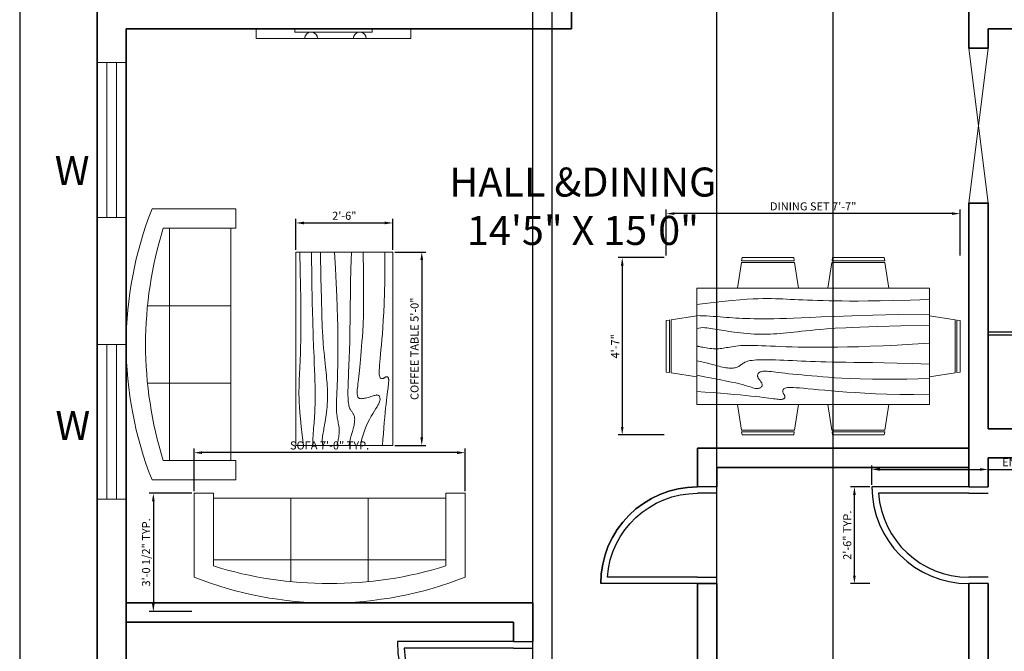
# Model space of a CAD drawing. Units: inches. Extents: x 1868 to 2413, y 1522 to 2138.
# Tile 2 of 4: x 1902 to 2207, y 1727 to 1923. Entities that reach past the tile are written whole.
import ezdxf

# ---------------------------------------------------------------- set-up
doc = ezdxf.new("R2010")
doc.units = ezdxf.units.IN
for name, color, linetype, lineweight in [('A-ANNO-DIMS', 2, 'Continuous', 18), ('A-ANNO-TEXT', 7, 'Continuous', 18), ('A-AREA-IDEN', 7, 'Continuous', 25), ('A-DOOR', 3, 'Continuous', 25), ('A-EQPM', 8, 'Continuous', 18), ('A-FLOR-CASE', 8, 'Continuous', 25), ('A-FLOR-OPEN', 4, 'Continuous', 18), ('A-FURN', 8, 'Continuous', 18), ('A-GLAZ', 4, 'Continuous', 18), ('A-WALL', 7, 'Continuous', 35), ('C-PROP', 7, 'Continuous', 25)]:
    doc.layers.add(name, color=color, linetype=linetype, lineweight=lineweight)
doc.styles.get("Standard").update_dxf_attribs({"font": 'arial.ttf'})
doc.dimstyles.new('ISO-25', dxfattribs={"dimtxt": 2.5, "dimasz": 2.5, "dimexe": 1.25, "dimexo": 0.625, "dimtad": 1, "dimdec": 0, "dimlunit": 3, "dimtxsty": 'Standard', "dimcen": 2.5, "dimadec": 0, "dimazin": 0, "dimtfac": 1, "dimtdec": 0, "dimtmove": 0, "dimatfit": 3, "dimfxl": 1, "dimarcsym": 0})

# ---------------------------------------------------------------- blocks, each defined once
blk = doc.blocks.new('Sofa - Roundback 7 ft.')
for p, q in [((-12.00002, -32.4421), (-12.00003, -6.5971)), ((11.99997, -32.4421), (11.99998, -6.5971)), ((-36.000027, -34), (-36.000027, -11.4696)), ((35.99998, -34), (35.99998, -11.4696)), ((-35.999844, -13.3819), (35.9998, -13.3819)), ((-36.000027, -32.4421), (35.99998, -32.4421))]:
    blk.add_line(p, q)
for points in [[(-36.000027, -34), (-42.000027, -34), (-42.000027, -8)], [(41.99998, -8), (41.99998, -34), (35.99998, -34)]]:
    blk.add_lwpolyline(points)
for centre, radius, start, end in [((0, -114.25), 114.25, 68.43141, 111.5686), ((-0.00001, -127.1968), 121.1968, 72.72033, 107.2797)]:
    blk.add_arc(centre, radius, start, end)
blk = doc.blocks.new('Table - Rectangular Woodgrain 60 x 30 in.')
for p, q in [((0, 0), (0, -30)), ((60, 0), (0, 0)), ((60, -30), (60, 0)), ((0, -30), (60, -30))]:
    blk.add_line(p, q)
for points in [[(0, -2.4), (4.8155, -2.418), (9.0302, -2.4688), (12.709, -2.5477), (15.9167, -2.65), (18.7181, -2.7711), (21.1781, -2.9063), (23.3616, -3.0508), (25.3333, -3.2), (27.1477, -3.3495), (28.8172, -3.4958), (30.3437, -3.636), (31.7291, -3.7667), (32.9756, -3.8849), (34.0849, -3.9875), (35.059, -4.0714), (35.9, -4.1334), (36.6114, -4.1711), (37.2041, -4.1854), (37.6906, -4.1779), (38.0833, -4.15), (38.3948, -4.1034), (38.6375, -4.0396), (38.8239, -3.9602), (38.9666, -3.8667), (39.0764, -3.7608), (39.1573, -3.6448), (39.2116, -3.521), (39.2416, -3.3917), (39.2498, -3.2593), (39.2385, -3.1261), (39.21, -2.9944), (39.1666, -2.8667), (39.111, -2.7447), (39.0468, -2.6281), (38.978, -2.5163), (38.9083, -2.4083), (38.8418, -2.3035), (38.7823, -2.201), (38.7337, -2.1001), (38.7, -2), (38.6844, -1.9003), (38.6875, -1.8021), (38.7094, -1.707), (38.75, -1.6167), (38.8094, -1.5326), (38.8875, -1.4563), (38.9844, -1.3893), (39.1, -1.3333), (39.2351, -1.2896), (39.3937, -1.2583), (39.5804, -1.2396), (39.8, -1.2333), (40.057, -1.2396), (40.3562, -1.2583), (40.7023, -1.2896), (41.1, -1.3333), (41.5547, -1.3895), (42.0755, -1.4573), (42.6721, -1.5361), (43.3542, -1.625), (44.1316, -1.7233), (45.014, -1.8302), (46.0114, -1.9449), (47.1333, -2.0667), (48.3862, -2.1947), (49.7625, -2.3281), (51.2513, -2.4663), (52.8416, -2.6083), (54.5226, -2.7535), (56.2833, -2.9011), (58.1127, -3.0501), (60, -3.2)], [(0, -9.2), (6.5759, -9.0858), (11.9385, -9.0365), (16.2527, -9.0418), (19.6833, -9.0917), (22.3952, -9.1759), (24.5531, -9.2844), (26.322, -9.4069), (27.8666, -9.5333), (29.3241, -9.6553), (30.7203, -9.7719), (32.0532, -9.8837), (33.3208, -9.9917), (34.5213, -10.0965), (35.6526, -10.199), (36.7128, -10.2999), (37.7, -10.4), (38.6129, -10.4996), (39.4531, -10.5969), (40.223, -10.6895), (40.925, -10.775), (41.5613, -10.8512), (42.1344, -10.9156), (42.6465, -10.966), (43.1, -11), (43.4976, -11.0158), (43.8437, -11.0136), (44.143, -10.9942), (44.4, -10.9583), (44.6195, -10.9069), (44.8062, -10.8406), (44.9648, -10.7603), (45.1, -10.6667), (45.2155, -10.5598), (45.3114, -10.4365), (45.3871, -10.2929), (45.4416, -10.125), (45.4743, -9.929), (45.4844, -9.7011), (45.4709, -9.4371), (45.4333, -9.1333), (45.3716, -8.7883), (45.2896, -8.4104), (45.1919, -8.0107), (45.0833, -7.6), (44.9685, -7.1893), (44.8521, -6.7896), (44.7388, -6.4117), (44.6333, -6.0667), (44.54, -5.7628), (44.4614, -5.4979), (44.4001, -5.2675), (44.3583, -5.0667), (44.3384, -4.8909), (44.3427, -4.7354), (44.3736, -4.5956), (44.4333, -4.4667), (44.5236, -4.3453), (44.6427, -4.2333), (44.7884, -4.1339), (44.9583, -4.05), (45.1501, -3.9849), (45.3614, -3.9417), (45.59, -3.9234), (45.8333, -3.9333), (46.0915, -3.9749), (46.3734, -4.0531), (46.6906, -4.1736), (47.0542, -4.3417), (47.4756, -4.5629), (47.9661, -4.8427), (48.5372, -5.1866), (49.2, -5.6), (49.9676, -6.0844), (50.8594, -6.625), (51.8965, -7.2031), (53.1, -7.8), (54.491, -8.3969), (56.0906, -8.975), (57.9199, -9.5156), (60, -10)], [(0, -12.8), (5.1847, -12.9322), (9.6213, -13.0323), (13.3963, -13.1059), (16.5958, -13.1583), (19.3063, -13.1952), (21.614, -13.2219), (23.6054, -13.2439), (25.3666, -13.2667), (26.9728, -13.2947), (28.4531, -13.3281), (29.8256, -13.3663), (31.1083, -13.4083), (32.3191, -13.4535), (33.476, -13.501), (34.597, -13.5501), (35.7, -13.6), (36.7984, -13.6497), (37.8875, -13.6979), (38.9578, -13.743), (40, -13.7833), (41.0047, -13.8174), (41.9625, -13.8438), (42.864, -13.8607), (43.7, -13.8667), (44.4631, -13.8604), (45.1552, -13.8417), (45.7801, -13.8104), (46.3416, -13.7667), (46.8439, -13.7104), (47.2906, -13.6417), (47.6858, -13.5604), (48.0333, -13.4667), (48.3375, -13.3608), (48.6042, -13.2448), (48.8396, -13.121), (49.05, -12.9917), (49.2417, -12.8593), (49.4208, -12.7261), (49.5937, -12.5944), (49.7667, -12.4667), (49.9452, -12.3451), (50.1323, -12.2313), (50.3303, -12.1268), (50.5416, -12.0333), (50.7686, -11.9524), (51.0135, -11.8854), (51.2788, -11.8341), (51.5666, -11.8), (51.8785, -11.7843), (52.2116, -11.7865), (52.562, -11.8059), (52.926, -11.8417), (53.2998, -11.8931), (53.6795, -11.9594), (54.0614, -12.0397), (54.4416, -12.1333), (54.8223, -12.2401), (55.2293, -12.3625), (55.6942, -12.5037), (56.2489, -12.6667), (56.9251, -12.8547), (57.7545, -13.0708), (58.7689, -13.3182), (60, -13.6)], [(0, -18), (5.124, -17.7273), (9.6609, -17.5057), (13.6705, -17.3303), (17.2125, -17.1958), (20.3467, -17.0973), (23.1328, -17.0297), (25.6307, -16.9878), (27.9, -16.9667), (29.9928, -16.9617), (31.9302, -16.9703), (33.7254, -16.9907), (35.3917, -17.0208), (36.9423, -17.0588), (38.3906, -17.1026), (39.7499, -17.1503), (41.0333, -17.2), (42.2519, -17.2496), (43.4073, -17.2969), (44.4986, -17.3395), (45.525, -17.375), (46.4858, -17.4012), (47.3802, -17.4156), (48.2074, -17.416), (48.9667, -17.4), (49.6583, -17.3662), (50.2872, -17.3167), (50.8595, -17.2547), (51.3812, -17.1833), (51.8584, -17.1057), (52.2971, -17.025), (52.7034, -16.9443), (53.0833, -16.8667), (53.443, -16.7951), (53.789, -16.7313), (54.128, -16.6768), (54.4666, -16.6334), (54.8115, -16.6024), (55.1693, -16.5854), (55.5465, -16.5841), (55.95, -16.6), (56.3828, -16.6337), (56.8346, -16.6823), (57.2915, -16.7418), (57.7396, -16.8084), (58.165, -16.878), (58.5539, -16.9469), (58.8924, -17.0111), (59.1666, -17.0667), (59.3679, -17.1107), (59.5078, -17.1438), (59.6032, -17.1675), (59.6708, -17.1833), (59.7275, -17.193), (59.7901, -17.1979), (59.8753, -17.1998), (60, -17.2)], [(0, -22.4), (8.0098, -22.2501), (14.4094, -22.1011), (19.4168, -21.9535), (23.25, -21.8083), (26.1269, -21.6663), (28.2656, -21.5281), (29.884, -21.3947), (31.2, -21.2667), (32.3967, -21.1448), (33.5172, -21.0292), (34.5697, -20.9198), (35.5625, -20.8167), (36.5037, -20.7198), (37.4015, -20.6292), (38.2642, -20.5448), (39.1, -20.4667), (39.9164, -20.3951), (40.7187, -20.3313), (41.5117, -20.2768), (42.3, -20.2333), (43.0883, -20.2024), (43.8812, -20.1854), (44.6836, -20.1841), (45.5, -20.2), (46.3328, -20.234), (47.1747, -20.2844), (48.0163, -20.3488), (48.8479, -20.425), (49.66, -20.5106), (50.4429, -20.6031), (51.1872, -20.7004), (51.8833, -20.8), (52.5246, -20.8999), (53.1166, -20.9995), (53.6681, -21.0983), (54.1875, -21.1958), (54.6834, -21.2919), (55.1646, -21.3859), (55.6394, -21.4777), (56.1167, -21.5667), (56.6028, -21.6515), (57.0961, -21.7266), (57.5929, -21.7852), (58.0896, -21.8208), (58.5823, -21.8268), (59.0674, -21.7964), (59.5412, -21.723), (60, -21.6)], [(0, -25.2), (8.6355, -25.0504), (15.7026, -24.9031), (21.4049, -24.7606), (25.9458, -24.625), (29.529, -24.4988), (32.3578, -24.3844), (34.6359, -24.284), (36.5667, -24.2), (38.3213, -24.1341), (39.9417, -24.0854), (41.437, -24.0523), (42.8167, -24.0333), (44.0901, -24.0268), (45.2667, -24.0313), (46.3557, -24.0451), (47.3667, -24.0667), (48.309, -24.0947), (49.1928, -24.1287), (50.0284, -24.168), (50.826, -24.2125), (51.5959, -24.2617), (52.3483, -24.3151), (53.0935, -24.3725), (53.8417, -24.4334), (54.6009, -24.497), (55.3699, -24.561), (56.1454, -24.6226), (56.9239, -24.6792), (57.7021, -24.7279), (58.4764, -24.7662), (59.2435, -24.7911), (60, -24.8)], [(0, -28.8), (5.6867, -28.6681), (10.45, -28.5698), (14.407, -28.5012), (17.675, -28.4584), (20.3711, -28.4374), (22.6125, -28.4344), (24.5164, -28.4455), (26.2, -28.4667), (27.762, -28.4947), (29.2276, -28.5281), (30.6033, -28.5663), (31.8958, -28.6084), (33.1118, -28.6535), (34.2578, -28.7011), (35.3405, -28.7501), (36.3666, -28.8), (37.3443, -28.8497), (38.288, -28.8974), (39.2137, -28.9412), (40.1375, -28.9792), (41.0753, -29.0093), (42.0432, -29.0297), (43.0572, -29.0384), (44.1333, -29.0333), (45.2936, -29.0114), (46.5843, -28.9641), (48.0579, -28.8816), (49.7666, -28.7542), (51.7629, -28.5721), (54.0989, -28.3255), (56.8272, -28.0048), (60, -27.6)]]:
    blk.add_lwpolyline(points)
blk = doc.blocks.new('Dining Set - 36 x 72 in.')
for p, q in [((-22, 27.5), (-22.1562, 26.50042)), ((-22, 27.5), (-6, 27.5)), ((-5.8437, 26.49966), (-6, 27.5)), ((6, 27.5), (5.8438, 26.50042)), ((6, 27.5), (22, 27.5)), ((22.1563, 26.49966), (22, 27.5)), ((-22.2343, 26.00059), (-23.4847, 17.99762)), ((-22.2304, 26), (-5.7608, 26)), ((-5.8416, 26.5), (-22.1534, 26.5)), ((-4.5152, 17.99762), (-5.7655, 25.99926)), ((5.7657, 26.00059), (4.5153, 17.99762)), ((5.7696, 26), (22.2392, 26)), ((22.1584, 26.5), (5.8466, 26.5)), ((23.4848, 17.99762), (22.2345, 25.99926)), ((36, 18), (-36, 18)), ((-36, 18), (-36, -18)), ((36, -18), (36, 18)), ((-44.0006, 8.23428), (-35.9976, 9.48474)), ((44.0006, 8.23428), (35.9976, 9.48474)), ((-45.5, 8), (-44.5004, 8.15617)), ((-45.5, 8), (-45.5, -8)), ((-44.5, -8.15843), (-44.5, 8.15338)), ((-44, 8.23041), (-44, -8.23915)), ((44, 8.23041), (44, -8.23915)), ((44.5, -8.15843), (44.5, 8.15338)), ((45.5, 8), (44.5005, 8.15617)), ((45.5, 8), (45.5, -8)), ((-44.4997, -8.15631), (-45.5, -8)), ((-35.9976, -9.48476), (-43.9993, -8.2345)), ((35.9976, -9.48476), (43.9993, -8.2345)), ((44.4997, -8.15631), (45.5, -8)), ((-36, -18), (36, -18)), ((-22.2343, -26.0006), (-23.4847, -17.99762)), ((-4.5152, -17.99762), (-5.7655, -25.99928)), ((5.7657, -26.0006), (4.5153, -17.99762)), ((23.4848, -17.99762), (22.2345, -25.99928)), ((-22.2304, -26), (-5.7608, -26)), ((-22, -27.5), (-22.1562, -26.50044)), ((-5.8416, -26.5), (-22.1534, -26.5)), ((-5.8437, -26.49967), (-6, -27.5)), ((5.7696, -26), (22.2392, -26)), ((6, -27.5), (5.8438, -26.50044)), ((22.1584, -26.5), (5.8466, -26.5)), ((22.1563, -26.49967), (22, -27.5)), ((-22, -27.5), (-6, -27.5)), ((6, -27.5), (22, -27.5))]:
    blk.add_line(p, q)
for points in [[(-36, 15), (-31.1772, 14.97754), (-26.8079, 14.91406), (-22.8538, 14.81543), (-19.276, 14.6875), (-16.0362, 14.53613), (-13.0957, 14.36718), (-10.4159, 14.18652), (-7.9583, 14), (-5.6904, 13.81315), (-3.6035, 13.63021), (-1.6954, 13.45508), (0.0365, 13.29166), (1.5945, 13.14388), (2.9811, 13.01562), (4.1988, 12.9108), (5.25, 12.83333), (6.1393, 12.78613), (6.8802, 12.76823), (7.4883, 12.77767), (7.9792, 12.8125), (8.3685, 12.87077), (8.6719, 12.95052), (8.9049, 13.0498), (9.0833, 13.16666), (9.2205, 13.29899), (9.3216, 13.44401), (9.3895, 13.59879), (9.4271, 13.76041), (9.4373, 13.92594), (9.4232, 14.09245), (9.3875, 14.257), (9.3333, 14.41666), (9.2638, 14.56917), (9.1836, 14.71484), (9.0975, 14.85465), (9.0104, 14.98958), (8.9272, 15.1206), (8.8529, 15.2487), (8.7922, 15.37483), (8.75, 15.5), (8.7305, 15.62467), (8.7344, 15.74739), (8.7617, 15.86621), (8.8125, 15.97916), (8.8867, 16.08431), (8.9844, 16.17968), (9.1055, 16.26334), (9.25, 16.33333), (9.4189, 16.38802), (9.6172, 16.42708), (9.8506, 16.45052), (10.125, 16.45833), (10.4463, 16.45052), (10.8203, 16.42708), (11.2529, 16.38802), (11.75, 16.33333), (12.3184, 16.26318), (12.9694, 16.17838), (13.7151, 16.07991), (14.5677, 15.96875), (15.5395, 15.84586), (16.6426, 15.71224), (17.8893, 15.56884), (19.2917, 15.41666), (20.859, 15.25667), (22.5879, 15.08984), (24.4721, 14.91715), (26.5052, 14.73958), (28.6809, 14.5581), (30.9929, 14.3737), (33.4347, 14.18733), (36, 14)], [(-36, 10), (-28.9766, 10.14274), (-23.1725, 10.20442), (-18.4241, 10.19775), (-14.5677, 10.13541), (-11.4399, 10.03011), (-8.877, 9.89453), (-6.7154, 9.74137), (-4.7917, 9.58333), (-2.9698, 9.43082), (-1.2246, 9.28515), (0.4415, 9.14534), (2.026, 9.01041), (3.5266, 8.87939), (4.9408, 8.7513), (6.266, 8.62516), (7.5, 8.5), (8.6411, 8.37549), (9.6914, 8.2539), (10.6538, 8.13818), (11.5312, 8.03125), (12.3267, 7.93603), (13.043, 7.85547), (13.6831, 7.79248), (14.25, 7.75), (14.7471, 7.7303), (15.1797, 7.73307), (15.5537, 7.75732), (15.875, 7.80208), (16.1494, 7.86637), (16.3828, 7.94922), (16.5811, 8.04964), (16.75, 8.16666), (16.8944, 8.29915), (17.0143, 8.44531), (17.1089, 8.60319), (17.1771, 8.77083), (17.218, 8.94629), (17.2305, 9.1276), (17.2137, 9.31282), (17.1667, 9.5), (17.0895, 9.6875), (16.987, 9.875), (16.8649, 10.0625), (16.7292, 10.25), (16.5856, 10.4375), (16.4401, 10.625), (16.2985, 10.8125), (16.1667, 11), (16.05, 11.18733), (15.9518, 11.3737), (15.8752, 11.5581), (15.8229, 11.73958), (15.798, 11.91715), (15.8034, 12.08984), (15.842, 12.25667), (15.9167, 12.41666), (16.0295, 12.56836), (16.1784, 12.70833), (16.3605, 12.83268), (16.5729, 12.9375), (16.8127, 13.01888), (17.0768, 13.07291), (17.3625, 13.0957), (17.6667, 13.08333), (17.9894, 13.03312), (18.3418, 12.94726), (18.7382, 12.82918), (19.1927, 12.68229), (19.7195, 12.51001), (20.3327, 12.31575), (21.0465, 12.10294), (21.875, 11.875), (22.8357, 11.63354), (23.959, 11.37304), (25.2786, 11.08618), (26.8282, 10.76562), (28.6414, 10.40405), (30.752, 9.99414), (33.1936, 9.52856), (36, 9)], [(-36, 5.5), (-30.7157, 5.3348), (-26.069, 5.20963), (-21.9946, 5.11767), (-18.4271, 5.05208), (-15.3009, 5.00602), (-12.5508, 4.97265), (-10.1112, 4.94515), (-7.9167, 4.91666), (-5.909, 4.88167), (-4.0586, 4.83984), (-2.3429, 4.79215), (-0.7396, 4.73958), (0.7739, 4.6831), (2.22, 4.6237), (3.6213, 4.56233), (5, 4.5), (6.373, 4.43782), (7.7344, 4.3776), (9.0723, 4.32129), (10.375, 4.27083), (11.6309, 4.22819), (12.8281, 4.19531), (13.9551, 4.17415), (15, 4.16666), (15.954, 4.17448), (16.819, 4.19791), (17.6001, 4.23698), (18.3021, 4.29166), (18.9299, 4.36198), (19.4883, 4.44791), (19.9823, 4.54948), (20.4167, 4.66666), (20.7969, 4.79899), (21.1302, 4.94401), (21.4245, 5.09879), (21.6875, 5.26041), (21.9271, 5.42594), (22.1511, 5.59245), (22.3672, 5.757), (22.5834, 5.91666), (22.8065, 6.06868), (23.0404, 6.21093), (23.2879, 6.34147), (23.5521, 6.45833), (23.8358, 6.55957), (24.142, 6.64323), (24.4735, 6.70735), (24.8334, 6.75), (25.2235, 6.76969), (25.642, 6.76692), (26.0858, 6.74267), (26.5521, 6.69791), (27.0379, 6.63362), (27.5404, 6.55078), (28.0565, 6.45036), (28.5834, 6.33333), (29.1242, 6.19987), (29.7071, 6.04687), (30.3661, 5.87044), (31.1354, 5.66666), (32.0493, 5.43164), (33.142, 5.16146), (34.4475, 4.85221), (36, 4.5)], [(-36, -1), (-30.7915, -0.6591), (-26.0195, -0.38216), (-21.6519, -0.16284), (-17.6563, 0.00521), (-14.0005, 0.12833), (-10.6523, 0.21289), (-7.5796, 0.26522), (-4.75, 0.29166), (-2.134, 0.29793), (0.2878, 0.28711), (2.5317, 0.26163), (4.6146, 0.22396), (6.5529, 0.17651), (8.3633, 0.12174), (10.0623, 0.06209), (11.6667, 0), (13.1899, -0.06201), (14.6341, -0.1211), (15.9982, -0.17432), (17.2813, -0.21875), (18.4823, -0.25147), (19.6003, -0.26953), (20.6343, -0.27002), (21.5834, -0.25), (22.4481, -0.20768), (23.2357, -0.14584), (23.9549, -0.06836), (24.6146, 0.02083), (25.2235, 0.11784), (25.7904, 0.21875), (26.3241, 0.31966), (26.8334, 0.41666), (27.3265, 0.50618), (27.8099, 0.58593), (28.2894, 0.65397), (28.7709, 0.70833), (29.2601, 0.74707), (29.763, 0.76823), (30.2855, 0.76985), (30.8334, 0.75), (31.4088, 0.70784), (31.9994, 0.64713), (32.589, 0.57275), (33.1615, 0.48958), (33.7008, 0.4025), (34.1908, 0.3164), (34.6153, 0.23616), (34.9584, 0.16666), (35.2099, 0.11165), (35.3848, 0.07031), (35.504, 0.04069), (35.5886, 0.02083), (35.6594, 0.00879), (35.7377, 0.0026), (35.8442, 0.00032), (36, 0)], [(-36, -6.5), (-27.1843, -6.31267), (-20.084, -6.1263), (-14.469, -5.9419), (-10.1094, -5.76042), (-6.7752, -5.58285), (-4.2363, -5.41016), (-2.2629, -5.24333), (-0.625, -5.08334), (0.8708, -4.93099), (2.2715, -4.78646), (3.5872, -4.64974), (4.8281, -4.52084), (6.0046, -4.39974), (7.127, -4.28646), (8.2053, -4.18099), (9.25, -4.08334), (10.2705, -3.99382), (11.2734, -3.91407), (12.2647, -3.84603), (13.25, -3.79167), (14.2354, -3.75293), (15.2266, -3.73177), (16.2295, -3.73015), (17.25, -3.75), (18.2912, -3.79248), (19.3451, -3.85547), (20.4009, -3.93604), (21.4479, -4.03125), (22.4754, -4.13819), (23.4727, -4.25391), (24.4289, -4.37549), (25.3334, -4.5), (26.1785, -4.62492), (26.9694, -4.74935), (27.7145, -4.87281), (28.4219, -4.99479), (29.1, -5.11483), (29.7572, -5.23242), (30.4016, -5.34709), (31.0417, -5.45834), (31.6837, -5.56437), (32.3262, -5.65821), (32.9658, -5.73153), (33.599, -5.77604), (34.2224, -5.78345), (34.8327, -5.74545), (35.4264, -5.65373), (36, -5.5)], [(-36, -10), (-26.4022, -9.81299), (-18.4675, -9.62891), (-11.9839, -9.45069), (-6.7396, -9.28125), (-2.5226, -9.12354), (0.8789, -8.98047), (3.6769, -8.85498), (6.0833, -8.75), (8.2767, -8.66765), (10.3021, -8.60677), (12.1712, -8.56543), (13.8958, -8.54167), (15.4876, -8.53353), (16.9583, -8.53907), (18.3197, -8.55632), (19.5834, -8.58334), (20.7616, -8.61841), (21.8685, -8.66081), (22.9188, -8.71004), (23.9271, -8.76563), (24.9081, -8.82707), (25.8763, -8.89388), (26.8465, -8.96558), (27.8334, -9.04167), (28.8474, -9.12118), (29.8828, -9.20117), (30.93, -9.27824), (31.9792, -9.34896), (33.0205, -9.40991), (34.0443, -9.45768), (35.0407, -9.48885), (36, -9.5)], [(-36, -14.5), (-30.0881, -14.33513), (-25.0332, -14.21224), (-20.7312, -14.12647), (-17.0781, -14.07292), (-13.97, -14.04671), (-11.3027, -14.04297), (-8.9724, -14.05681), (-6.875, -14.08334), (-4.9224, -14.11833), (-3.0905, -14.16016), (-1.3709, -14.20785), (0.2448, -14.26042), (1.7647, -14.3169), (3.1973, -14.3763), (4.5507, -14.43767), (5.8333, -14.5), (7.0554, -14.5621), (8.235, -14.62175), (9.3922, -14.67652), (10.5469, -14.72396), (11.7192, -14.76164), (12.929, -14.78711), (14.1965, -14.79794), (15.5417, -14.79167), (16.9933, -14.76424), (18.6152, -14.70508), (20.4804, -14.60197), (22.6615, -14.44271), (25.2312, -14.21509), (28.2624, -13.9069), (31.8277, -13.50594), (36, -13)]]:
    blk.add_lwpolyline(points)
blk = doc.blocks.new('WIN-48IN')
for p, q in [((0, 48), (0, 0)), ((9, 48), (0, 48)), ((3, 48), (3, 0)), ((6, 0), (6, 48)), ((9, 0), (9, 48)), ((0, 0), (9, 0))]:
    blk.add_line(p, q)
blk = doc.blocks.new('DOOR-36IN')
for p, q in [((36, 36), (0, 36)), ((0.06, 34), (0, 34)), ((36, 34), (2.06, 34)), ((36, 36), (42, 36)), ((36, 34), (42, 34)), ((42, 2), (36, 2)), ((42, 0), (36, 0))]:
    blk.add_line(p, q)
for radius, start in [(36, 180), (34, 183.3723)]:
    blk.add_arc((36, 36), radius, start, 270)
blk = doc.blocks.new('DOOR-30IN')
for p, q in [((30, 30), (0, 30)), ((0.07, 28), (0, 28)), ((30, 28), (2.07, 28)), ((30, 30), (36, 30)), ((30, 28), (36, 28)), ((36, 2), (30, 2)), ((36, 0), (30, 0))]:
    blk.add_line(p, q)
for radius, start in [(30, 180), (28, 184.096)]:
    blk.add_arc((30, 30), radius, start, 270)
blk = doc.blocks.new('*D32')
at = {"layer": 'A-ANNO-DIMS', "color": 0, "lineweight": -2, "transparency": 16777216}
for p, q in [((2166.46, 1778.58), (2166.46, 1784.6)), ((2202.46, 1778.58), (2202.46, 1784.6)), ((2168.96, 1783.35), (2199.96, 1783.35)), ((2202.46, 1783.35), (2245.57, 1783.35))]:
    blk.add_line(p, q, dxfattribs=at)
at = {"layer": 'A-ANNO-DIMS', "color": 0, "transparency": 16777216}
for points in [[(2168.96, 1783.77), (2168.96, 1782.93), (2166.46, 1783.35)], [(2199.96, 1783.77), (2199.96, 1782.93), (2202.46, 1783.35)]]:
    blk.add_solid(points, dxfattribs=at)
at = {"layer": 'Defpoints', "color": 0, "transparency": 16777216}
for p in [(2202.46, 1783.35), (2166.46, 1777.95), (2202.46, 1777.95)]:
    blk.add_point(p, dxfattribs=at)
at = {"layer": 'A-ANNO-DIMS', "color": 0, "transparency": 16777216, "insert": (2225.26, 1785.27), "char_height": 2.5, "attachment_point": 5}
blk.add_mtext('ENTRY DOOR 3\'-0" TYP.', dxfattribs=at)
blk = doc.blocks.new('*D33')
at = {"layer": 'A-ANNO-DIMS', "color": 0, "lineweight": -2, "transparency": 16777216}
for p, q in [((2165.83, 1777.95), (2159.81, 1777.95)), ((2161.06, 1750.45), (2161.06, 1775.45)), ((2165.83, 1747.95), (2159.81, 1747.95))]:
    blk.add_line(p, q, dxfattribs=at)
at = {"layer": 'A-ANNO-DIMS', "color": 0, "transparency": 16777216}
for points in [[(2160.64, 1775.45), (2161.47, 1775.45), (2161.06, 1777.95)], [(2160.64, 1750.45), (2161.47, 1750.45), (2161.06, 1747.95)]]:
    blk.add_solid(points, dxfattribs=at)
at = {"layer": 'Defpoints', "color": 0, "transparency": 16777216}
for p in [(2161.06, 1777.95), (2166.46, 1777.95), (2166.46, 1747.95)]:
    blk.add_point(p, dxfattribs=at)
at = {"layer": 'A-ANNO-DIMS', "color": 0, "transparency": 16777216, "insert": (2159.16, 1762.95), "char_height": 2.5, "attachment_point": 5, "rotation": 90}
blk.add_mtext('2\'-6" TYP.', dxfattribs=at)
blk = doc.blocks.new('*D42')
at = {"layer": 'A-ANNO-DIMS', "color": 0, "lineweight": -2, "transparency": 16777216}
for p, q in [((1956.46, 1776.58), (1956.46, 1789.8)), ((2037.96, 1788.55), (1958.96, 1788.55)), ((2040.46, 1776.58), (2040.46, 1789.8))]:
    blk.add_line(p, q, dxfattribs=at)
at = {"layer": 'A-ANNO-DIMS', "color": 0, "transparency": 16777216}
for points in [[(1958.96, 1788.97), (1958.96, 1788.13), (1956.46, 1788.55)], [(2037.96, 1788.97), (2037.96, 1788.13), (2040.46, 1788.55)]]:
    blk.add_solid(points, dxfattribs=at)
at = {"layer": 'Defpoints', "color": 0, "transparency": 16777216}
for p in [(1956.46, 1788.55), (1956.46, 1775.95), (2040.46, 1775.95)]:
    blk.add_point(p, dxfattribs=at)
at = {"layer": 'A-ANNO-DIMS', "color": 0, "transparency": 16777216, "insert": (1998.46, 1790.47), "char_height": 2.5, "attachment_point": 5}
blk.add_mtext('SOFA 7\'-0" TYP.', dxfattribs=at)
blk = doc.blocks.new('*D43')
at = {"layer": 'A-ANNO-DIMS', "color": 0, "lineweight": -2, "transparency": 16777216}
for p, q in [((1955.83, 1775.95), (1942.61, 1775.95)), ((1943.86, 1773.45), (1943.86, 1741.78)), ((1955.83, 1739.28), (1942.61, 1739.28))]:
    blk.add_line(p, q, dxfattribs=at)
at = {"layer": 'A-ANNO-DIMS', "color": 0, "transparency": 16777216}
for points in [[(1943.44, 1773.45), (1944.27, 1773.45), (1943.86, 1775.95)], [(1943.44, 1741.78), (1944.27, 1741.78), (1943.86, 1739.28)]]:
    blk.add_solid(points, dxfattribs=at)
at = {"layer": 'Defpoints', "color": 0, "transparency": 16777216}
for p in [(1956.46, 1775.95), (1943.86, 1739.28), (1956.46, 1739.28)]:
    blk.add_point(p, dxfattribs=at)
at = {"layer": 'A-ANNO-DIMS', "color": 0, "transparency": 16777216, "insert": (1941.94, 1757.62), "char_height": 2.5, "attachment_point": 5, "rotation": 90}
blk.add_mtext('3\'-0 1/2" TYP.', dxfattribs=at)
blk = doc.blocks.new('*D48')
at = {"layer": 'A-ANNO-DIMS', "color": 0, "lineweight": -2, "transparency": 16777216}
for p, q in [((2018.64, 1850.77), (2028.27, 1850.77)), ((2027.02, 1848.27), (2027.02, 1793.27)), ((2018.64, 1790.77), (2028.27, 1790.77))]:
    blk.add_line(p, q, dxfattribs=at)
at = {"layer": 'A-ANNO-DIMS', "color": 0, "transparency": 16777216}
for points in [[(2026.6, 1848.27), (2027.44, 1848.27), (2027.02, 1850.77)], [(2026.6, 1793.27), (2027.44, 1793.27), (2027.02, 1790.77)]]:
    blk.add_solid(points, dxfattribs=at)
at = {"layer": 'Defpoints', "color": 0, "transparency": 16777216}
for p in [(2018.02, 1850.77), (2018.02, 1790.77), (2027.02, 1790.77)]:
    blk.add_point(p, dxfattribs=at)
at = {"layer": 'A-ANNO-DIMS', "color": 0, "transparency": 16777216, "insert": (2025.1, 1820.77), "char_height": 2.5, "attachment_point": 5, "rotation": 90}
blk.add_mtext('COFFEE TABLE 5\'-0"', dxfattribs=at)
blk = doc.blocks.new('*D49')
at = {"layer": 'A-ANNO-DIMS', "color": 0, "lineweight": -2, "transparency": 16777216}
for p, q in [((1988.02, 1851.4), (1988.02, 1861.02)), ((2018.02, 1851.4), (2018.02, 1861.02)), ((1990.52, 1859.77), (2015.52, 1859.77))]:
    blk.add_line(p, q, dxfattribs=at)
at = {"layer": 'A-ANNO-DIMS', "color": 0, "transparency": 16777216}
for points in [[(1990.52, 1860.19), (1990.52, 1859.36), (1988.02, 1859.77)], [(2015.52, 1860.19), (2015.52, 1859.36), (2018.02, 1859.77)]]:
    blk.add_solid(points, dxfattribs=at)
at = {"layer": 'Defpoints', "color": 0, "transparency": 16777216}
for p in [(2018.02, 1859.77), (1988.02, 1850.77), (2018.02, 1850.77)]:
    blk.add_point(p, dxfattribs=at)
at = {"layer": 'A-ANNO-DIMS', "color": 0, "transparency": 16777216, "insert": (2003.02, 1861.68), "char_height": 2.5, "attachment_point": 5}
blk.add_mtext('2\'-6"', dxfattribs=at)
blk = doc.blocks.new('*D50')
at = {"layer": 'A-ANNO-DIMS', "color": 0, "lineweight": -2, "transparency": 16777216}
for p, q in [((2102.78, 1849.65), (2102.78, 1863.93)), ((2193.78, 1849.65), (2193.78, 1863.93)), ((2191.28, 1862.68), (2105.28, 1862.68))]:
    blk.add_line(p, q, dxfattribs=at)
at = {"layer": 'A-ANNO-DIMS', "color": 0, "transparency": 16777216}
for points in [[(2105.28, 1863.09), (2105.28, 1862.26), (2102.78, 1862.68)], [(2191.28, 1863.09), (2191.28, 1862.26), (2193.78, 1862.68)]]:
    blk.add_solid(points, dxfattribs=at)
at = {"layer": 'Defpoints', "color": 0, "transparency": 16777216}
for p in [(2102.78, 1862.68), (2102.78, 1849.03), (2193.78, 1849.03)]:
    blk.add_point(p, dxfattribs=at)
at = {"layer": 'A-ANNO-DIMS', "color": 0, "transparency": 16777216, "insert": (2148.28, 1864.6), "char_height": 2.5, "attachment_point": 5}
blk.add_mtext('DINING SET 7\'-7"', dxfattribs=at)
blk = doc.blocks.new('*D51')
at = {"layer": 'A-ANNO-DIMS', "color": 0, "lineweight": -2, "transparency": 16777216}
for p, q in [((2102.16, 1849.03), (2087.88, 1849.03)), ((2089.13, 1846.53), (2089.13, 1796.53)), ((2102.16, 1794.03), (2087.88, 1794.03))]:
    blk.add_line(p, q, dxfattribs=at)
at = {"layer": 'A-ANNO-DIMS', "color": 0, "transparency": 16777216}
for points in [[(2088.72, 1846.53), (2089.55, 1846.53), (2089.13, 1849.03)], [(2088.72, 1796.53), (2089.55, 1796.53), (2089.13, 1794.03)]]:
    blk.add_solid(points, dxfattribs=at)
at = {"layer": 'Defpoints', "color": 0, "transparency": 16777216}
for p in [(2102.78, 1849.03), (2089.13, 1794.03), (2102.78, 1794.03)]:
    blk.add_point(p, dxfattribs=at)
at = {"layer": 'A-ANNO-DIMS', "color": 0, "transparency": 16777216, "insert": (2087.26, 1821.53), "char_height": 2.5, "attachment_point": 5, "rotation": 90}
blk.add_mtext('4\'-7"', dxfattribs=at)
blk = doc.blocks.new('*D54')
at = {"layer": 'A-ANNO-DIMS', "color": 0, "lineweight": -2, "transparency": 16777216}
for p, q in [((2118.46, 1706.58), (2118.46, 2135.38)), ((2154.46, 1706.58), (2154.46, 2135.38)), ((2120.96, 2134.13), (2151.96, 2134.13))]:
    blk.add_line(p, q, dxfattribs=at)
at = {"layer": 'A-ANNO-DIMS', "color": 0, "transparency": 16777216}
for points in [[(2120.96, 2134.54), (2120.96, 2133.71), (2118.46, 2134.13)], [(2151.96, 2134.54), (2151.96, 2133.71), (2154.46, 2134.13)]]:
    blk.add_solid(points, dxfattribs=at)
at = {"layer": 'Defpoints', "color": 0, "transparency": 16777216}
for p in [(2154.46, 2134.13), (2118.46, 1705.95), (2154.46, 1705.95)]:
    blk.add_point(p, dxfattribs=at)
at = {"layer": 'A-ANNO-DIMS', "color": 0, "transparency": 16777216, "insert": (2136.46, 2136.03), "char_height": 2.5, "attachment_point": 5}
blk.add_mtext('3\'-0"', dxfattribs=at)
blk = doc.blocks.new('*D61')
at = {"layer": 'A-ANNO-DIMS', "color": 0, "lineweight": -2, "transparency": 16777216}
for p, q in [((2061.46, 1682.58), (2061.46, 2135.38)), ((2067.46, 1682.58), (2067.46, 2135.38)), ((2058.96, 2134.13), (2056.46, 2134.13)), ((2061.46, 2134.13), (2067.46, 2134.13)), ((2069.96, 2134.13), (2080.35, 2134.13))]:
    blk.add_line(p, q, dxfattribs=at)
at = {"layer": 'A-ANNO-DIMS', "color": 0, "transparency": 16777216}
for points in [[(2058.96, 2134.54), (2058.96, 2133.71), (2061.46, 2134.13)], [(2069.96, 2134.54), (2069.96, 2133.71), (2067.46, 2134.13)]]:
    blk.add_solid(points, dxfattribs=at)
at = {"layer": 'Defpoints', "color": 0, "transparency": 16777216}
for p in [(2067.46, 2134.13), (2061.46, 1681.95), (2067.46, 1681.95)]:
    blk.add_point(p, dxfattribs=at)
at = {"layer": 'A-ANNO-DIMS', "color": 0, "transparency": 16777216, "insert": (2076.4, 2136.03), "char_height": 2.5, "attachment_point": 5}
blk.add_mtext('0\'-6"', dxfattribs=at)

msp = doc.modelspace()

# ---------------------------------------------------------------- linework, layer by layer
at = {"layer": 'A-DOOR'}
msp.add_line((2118.46, 1747.95), (2112.46, 1747.95), dxfattribs=at)
msp.add_arc((2112.46, 1747.95), 30, 90, 180, dxfattribs=at)
at = {"layer": 'A-EQPM'}
for p, q in [((1975.67, 1919.95), (1975.67, 1916.95)), ((1975.67, 1919.95), (2023.67, 1919.95)), ((1975.67, 1919.95), (1987.67, 1919.95)), ((1987.67, 1919.95), (1987.67, 1918.95)), ((2011.67, 1918.95), (1987.67, 1918.95)), ((2023.67, 1919.95), (2011.67, 1919.95)), ((2011.67, 1919.95), (2011.67, 1918.95)), ((2023.67, 1916.95), (2023.67, 1919.95)), ((1975.67, 1916.95), (2023.67, 1916.95))]:
    msp.add_line(p, q, dxfattribs=at)
for centre in [(1992.74, 1916.95), (2007.82, 1916.95)]:
    msp.add_arc(centre, 2, 0, 180, dxfattribs=at)
at = {"layer": 'A-FLOR-CASE'}
for p, q in [((2317.46, 1825.95), (2202.46, 1825.95)), ((2317.46, 1824.95), (2202.46, 1824.95))]:
    msp.add_line(p, q, dxfattribs=at)
at = {"layer": 'A-FLOR-OPEN'}
for p, q in [((2196.46, 1865.95), (2202.46, 1913.95)), ((2202.46, 1913.95), (2196.46, 1913.95)), ((2196.46, 1913.95), (2202.46, 1865.95))]:
    msp.add_line(p, q, dxfattribs=at)
at = {"layer": 'A-WALL'}
for p, q in [((1926.46, 2078.95), (1926.46, 1588.95)), ((2073.46, 1937.95), (2073.46, 1919.95)), ((2196.46, 1919.95), (2196.46, 1937.95)), ((2067.46, 1919.95), (1935.46, 1919.95)), ((1935.46, 1919.95), (1935.46, 1597.95)), ((2067.46, 1919.95), (2073.46, 1919.95)), ((2196.46, 1919.95), (2196.46, 1913.95)), ((2196.46, 1913.95), (2196.46, 1919.95)), ((2346.46, 1919.95), (2202.46, 1919.95)), ((2202.46, 1913.95), (2202.46, 1919.95)), ((2196.46, 1913.95), (2202.46, 1913.95)), ((2196.46, 1795.95), (2196.46, 1865.95)), ((2202.46, 1865.95), (2196.46, 1865.95)), ((2202.46, 1795.95), (2202.46, 1865.95)), ((2196.46, 1795.95), (2196.46, 1789.95)), ((2346.46, 1795.95), (2202.46, 1795.95)), ((2196.46, 1789.95), (2112.46, 1789.95)), ((2112.46, 1777.95), (2112.46, 1789.95)), ((2196.46, 1777.95), (2196.46, 1789.95)), ((2202.46, 1777.95), (2202.46, 1786.95)), ((2346.46, 1786.95), (2202.46, 1786.95)), ((2196.46, 1783.95), (2118.46, 1783.95)), ((2118.46, 1783.95), (2118.46, 1777.95)), ((2118.46, 1777.95), (2118.46, 1783.95)), ((2196.46, 1783.95), (2196.46, 1777.95)), ((2112.46, 1687.95), (2112.46, 1747.95)), ((2118.46, 1597.95), (2118.46, 1747.95)), ((2196.46, 1597.95), (2196.46, 1747.95)), ((2202.46, 1597.95), (2202.46, 1747.95)), ((1935.46, 1741.95), (2061.46, 1741.95)), ((2061.46, 1741.95), (2061.46, 1729.95)), ((1935.46, 1735.95), (2055.46, 1735.95)), ((2055.46, 1735.95), (2055.46, 1729.95)), ((2055.46, 1735.95), (2055.46, 1729.95))]:
    msp.add_line(p, q, dxfattribs=at)
at = {"layer": 'C-PROP'}
msp.add_line((1902.46, 2104.95), (1902.46, 1552.95), dxfattribs=at)

# ---------------------------------------------------------------- block references
at = {"layer": 'A-DOOR', "extrusion": (0, 0, -1), "zscale": -1, "rotation": 180}
msp.add_blockref('DOOR-30IN', (-2082.46, 1777.95), dxfattribs=at)
at = {"layer": 'A-DOOR'}
for name, p in [('DOOR-30IN', (2166.46, 1747.95)), ('DOOR-36IN', (2019.46, 1693.95))]:
    msp.add_blockref(name, p, dxfattribs=at)
at = {"layer": 'A-FURN'}
for name, p, rotation in [('Sofa - Roundback 7 ft.', (1935.46, 1822.11), 90), ('Table - Rectangular Woodgrain 60 x 30 in.', (2018.02, 1850.77), 270), ('Dining Set - 36 x 72 in.', (2148.28, 1821.53), 180), ('Sofa - Roundback 7 ft.', (1998.46, 1741.95), 180)]:
    msp.add_blockref(name, p, dxfattribs=dict(at, rotation=rotation))
at = {"layer": 'A-GLAZ'}
for p in [(1926.46, 1861.49), (1926.46, 1774.11)]:
    msp.add_blockref('WIN-48IN', p, dxfattribs=at)

# ---------------------------------------------------------------- texts
at = {"layer": 'A-ANNO-TEXT', "char_height": 9, "attachment_point": 1}
for insert in [(1876.8, 1880.55), (1877.02, 1801.5)]:
    msp.add_mtext_dynamic_manual_height_columns('\\pxqc;W', width=83.7859, gutter_width=12.5, heights=[0], dxfattribs=dict(at, insert=insert))
at = {"layer": 'A-AREA-IDEN', "insert": (2030.73, 1876.96), "char_height": 9, "attachment_point": 1}
msp.add_mtext_dynamic_manual_height_columns('\\pxqc;HALL &DINING\\P14\'5" X 15\'0"', width=92.4426, gutter_width=12.5, heights=[0], dxfattribs=at)

# ---------------------------------------------------------------- dimensions: what is measured, and where the dimension line sits
at = {"layer": 'A-ANNO-DIMS'}
for base, p1, p2, picture, middle in [((2067.46, 2134.13), (2061.46, 1681.95), (2067.46, 1681.95), '*D61', (2076.4, 2136.03)), ((2154.46, 2134.13), (2118.46, 1705.95), (2154.46, 1705.95), '*D54', (2136.46, 2136.03)), ((2018.02, 1859.77), (1988.02, 1850.77), (2018.02, 1850.77), '*D49', (2003.02, 1861.68))]:
    dim = msp.add_linear_dim(base=base, p1=p1, p2=p2, dimstyle='ISO-25', override={"dimdec": 1, "dimlfac": 1, "dimrnd": 0, "dimzin": 1, "dimdsep": 46, "dimlunit": 4, "dimfrac": 2}, dxfattribs=at)
    dim.commit()
    dim.dimension.update_dxf_attribs({"geometry": picture, "text_midpoint": middle})
for base, p1, p2, angle, text, picture, middle in [((2102.78, 1862.68), (2193.78, 1849.03), (2102.78, 1849.03), 180, 'DINING SET <>', '*D50', (2148.28, 1864.6)), ((2027.02, 1790.77), (2018.02, 1850.77), (2018.02, 1790.77), 270, 'COFFEE TABLE <>', '*D48', (2025.1, 1820.77)), ((1956.46, 1788.55), (2040.46, 1775.95), (1956.46, 1775.95), 180, 'SOFA <> TYP.', '*D42', (1998.46, 1790.47)), ((1943.86, 1739.28), (1956.46, 1775.95), (1956.46, 1739.28), 270, '<> TYP.', '*D43', (1941.94, 1757.62)), ((2161.06, 1777.95), (2166.46, 1747.95), (2166.46, 1777.95), 90, '<> TYP.', '*D33', (2159.16, 1762.95))]:
    dim = msp.add_linear_dim(base=base, p1=p1, p2=p2, angle=angle, text=text, dimstyle='ISO-25', override={"dimdec": 1, "dimlfac": 1, "dimrnd": 0, "dimzin": 1, "dimdsep": 46, "dimlunit": 4, "dimfrac": 2}, dxfattribs=at)
    dim.commit()
    dim.dimension.update_dxf_attribs({"geometry": picture, "text_midpoint": middle})
dim = msp.add_linear_dim(base=(2089.13, 1794.03), p1=(2102.78, 1849.03), p2=(2102.78, 1794.03), angle=270, dimstyle='ISO-25', override={"dimdec": 1, "dimlfac": 1, "dimrnd": 0, "dimzin": 1, "dimdsep": 46, "dimlunit": 4, "dimfrac": 2}, dxfattribs=at)
dim.commit()
dim.dimension.update_dxf_attribs({"geometry": '*D51', "text_midpoint": (2087.26, 1821.53)})
dim = msp.add_linear_dim(base=(2202.46, 1783.35), p1=(2166.46, 1777.95), p2=(2202.46, 1777.95), text='ENTRY DOOR <> TYP.', dimstyle='ISO-25', override={"dimdec": 1, "dimlfac": 1, "dimrnd": 0, "dimzin": 1, "dimdsep": 46, "dimlunit": 4, "dimfrac": 2}, dxfattribs=at)
dim.commit()
dim.dimension.update_dxf_attribs({"geometry": '*D32', "text_midpoint": (2225.26, 1785.27)})

doc.saveas('drawing.dxf')
